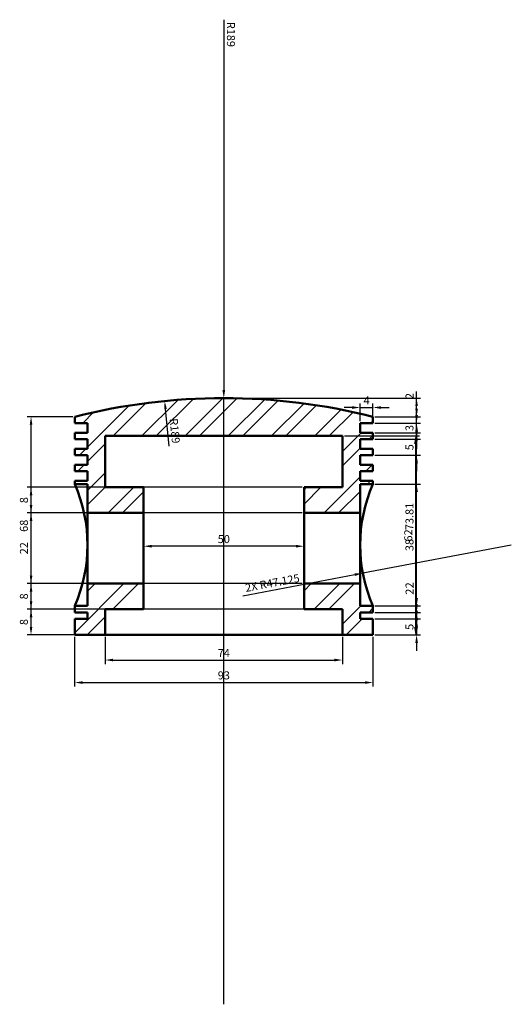
# Model space of a CAD drawing. Units: millimetres. Extents: x 2415 to 2568, y 1198 to 1505.
import ezdxf

# ---------------------------------------------------------------- set-up
doc = ezdxf.new("R2010")
doc.units = ezdxf.units.MM
doc.linetypes.add('CENTER', pattern=[50.8, 31.75, -6.35, 6.35, -6.35])
for name, color, linetype, lineweight in [('M-CNTR', 4, 'CENTER', 18), ('M-DIMS', 2, 'Continuous', 25), ('M-HATC', 8, 'Continuous', 18), ('M-OUTL', 7, 'Continuous', 50)]:
    doc.layers.add(name, color=color, linetype=linetype, lineweight=lineweight)
doc.styles.get("Standard").update_dxf_attribs({"font": 'arial.ttf'})
doc.dimstyles.new('ISO-25', dxfattribs={"dimtxt": 2.5, "dimasz": 2.5, "dimexe": 1.25, "dimexo": 0.625, "dimtad": 1, "dimtxsty": 'Standard', "dimcen": 2.5, "dimadec": 0, "dimazin": 0, "dimtfac": 1, "dimtmove": 0, "dimatfit": 3, "dimfxl": 1, "dimarcsym": 0})

# ---------------------------------------------------------------- blocks, each defined once
blk = doc.blocks.new('*D1')
at = {"layer": 'Defpoints', "color": 0, "transparency": 16777216}
for p in [(2431.97, 1313.29), (2524.97, 1313.29), (2524.97, 1298.42)]:
    blk.add_point(p, dxfattribs=at)
at = {"layer": 'M-DIMS', "color": 0, "lineweight": -2, "transparency": 16777216}
for p, q in [((2431.97, 1312.67), (2431.97, 1297.17)), ((2524.97, 1312.67), (2524.97, 1297.17)), ((2434.47, 1298.42), (2522.47, 1298.42))]:
    blk.add_line(p, q, dxfattribs=at)
at = {"layer": 'M-DIMS', "color": 0, "transparency": 16777216}
for points in [[(2434.47, 1298.84), (2434.47, 1298.01), (2431.97, 1298.42)], [(2522.47, 1298.84), (2522.47, 1298.01), (2524.97, 1298.42)]]:
    blk.add_solid(points, dxfattribs=at)
at = {"layer": 'M-DIMS', "color": 0, "transparency": 16777216, "insert": (2478.47, 1300.33), "char_height": 2.5, "attachment_point": 5}
blk.add_mtext('93', dxfattribs=at)
blk = doc.blocks.new('*D2')
at = {"layer": 'Defpoints', "color": 0, "transparency": 16777216}
for p in [(2441.47, 1313.29), (2515.47, 1313.29), (2515.47, 1305.44)]:
    blk.add_point(p, dxfattribs=at)
at = {"layer": 'M-DIMS', "color": 0, "lineweight": -2, "transparency": 16777216}
for p, q in [((2441.47, 1312.67), (2441.47, 1304.19)), ((2515.47, 1312.67), (2515.47, 1304.19)), ((2443.97, 1305.44), (2512.97, 1305.44))]:
    blk.add_line(p, q, dxfattribs=at)
at = {"layer": 'M-DIMS', "color": 0, "transparency": 16777216}
for points in [[(2443.97, 1305.86), (2443.97, 1305.02), (2441.47, 1305.44)], [(2512.97, 1305.86), (2512.97, 1305.02), (2515.47, 1305.44)]]:
    blk.add_solid(points, dxfattribs=at)
at = {"layer": 'M-DIMS', "color": 0, "transparency": 16777216, "insert": (2478.47, 1307.31), "char_height": 2.5, "attachment_point": 5}
blk.add_mtext('74', dxfattribs=at)
blk = doc.blocks.new('*D3')
at = {"layer": 'Defpoints', "color": 0, "transparency": 16777216}
for p in [(2453.47, 1359.29), (2503.47, 1359.29), (2453.47, 1340.92)]:
    blk.add_point(p, dxfattribs=at)
at = {"layer": 'M-DIMS', "color": 0, "lineweight": -2, "transparency": 16777216}
for p, q in [((2453.47, 1358.67), (2453.47, 1339.67)), ((2503.47, 1358.67), (2503.47, 1339.67)), ((2500.97, 1340.92), (2455.97, 1340.92))]:
    blk.add_line(p, q, dxfattribs=at)
at = {"layer": 'M-DIMS', "color": 0, "transparency": 16777216}
for points in [[(2455.97, 1341.34), (2455.97, 1340.5), (2453.47, 1340.92)], [(2500.97, 1341.34), (2500.97, 1340.5), (2503.47, 1340.92)]]:
    blk.add_solid(points, dxfattribs=at)
at = {"layer": 'M-DIMS', "color": 0, "transparency": 16777216, "insert": (2478.47, 1342.82), "char_height": 2.5, "attachment_point": 5}
blk.add_mtext('50', dxfattribs=at)
blk = doc.blocks.new('*D4')
at = {"layer": 'Defpoints', "color": 0, "transparency": 16777216}
for p in [(2515.47, 1375.29), (2524.97, 1313.29), (2538.21, 1313.29)]:
    blk.add_point(p, dxfattribs=at)
at = {"layer": 'M-DIMS', "color": 0, "lineweight": -2, "transparency": 16777216}
for p, q in [((2516.1, 1375.29), (2539.46, 1375.29)), ((2538.21, 1372.79), (2538.21, 1315.79)), ((2525.6, 1313.29), (2539.46, 1313.29))]:
    blk.add_line(p, q, dxfattribs=at)
at = {"layer": 'M-DIMS', "color": 0, "transparency": 16777216}
for points in [[(2537.79, 1372.79), (2538.62, 1372.79), (2538.21, 1375.29)], [(2537.79, 1315.79), (2538.62, 1315.79), (2538.21, 1313.29)]]:
    blk.add_solid(points, dxfattribs=at)
at = {"layer": 'M-DIMS', "color": 0, "transparency": 16777216, "insert": (2536.3, 1344.29), "char_height": 2.5, "attachment_point": 5, "rotation": 90}
blk.add_mtext('62', dxfattribs=at)
blk = doc.blocks.new('*D5')
at = {"layer": 'Defpoints', "color": 0, "transparency": 16777216}
for p in [(2524.97, 1384.17), (2520.97, 1379.29), (2524.97, 1379.29)]:
    blk.add_point(p, dxfattribs=at)
at = {"layer": 'M-DIMS', "color": 0, "lineweight": -2, "transparency": 16777216}
for p, q in [((2520.97, 1379.92), (2520.97, 1385.42)), ((2524.97, 1379.92), (2524.97, 1385.42)), ((2518.47, 1384.17), (2515.97, 1384.17)), ((2520.97, 1384.17), (2524.97, 1384.17)), ((2527.47, 1384.17), (2529.97, 1384.17))]:
    blk.add_line(p, q, dxfattribs=at)
at = {"layer": 'M-DIMS', "color": 0, "transparency": 16777216}
for points in [[(2518.47, 1384.58), (2518.47, 1383.75), (2520.97, 1384.17)], [(2527.47, 1384.58), (2527.47, 1383.75), (2524.97, 1384.17)]]:
    blk.add_solid(points, dxfattribs=at)
at = {"layer": 'M-DIMS', "color": 0, "transparency": 16777216, "insert": (2522.97, 1386.04), "char_height": 2.5, "attachment_point": 5}
blk.add_mtext('4', dxfattribs=at)
blk = doc.blocks.new('*D6')
at = {"layer": 'Defpoints', "color": 0, "transparency": 16777216}
for p in [(2460.04, 1386.2), (2478.47, 1198.1)]:
    blk.add_point(p, dxfattribs=at)
at = {"layer": 'M-DIMS', "color": 0, "lineweight": -2, "transparency": 16777216}
blk.add_line((2461.42, 1372.1), (2460.29, 1383.71), dxfattribs=at)
at = {"layer": 'M-DIMS', "color": 0, "transparency": 16777216}
blk.add_solid([(2460.7, 1383.75), (2459.87, 1383.67), (2460.04, 1386.2)], dxfattribs=at)
at = {"layer": 'M-DIMS', "color": 0, "transparency": 16777216, "insert": (2462.87, 1376.85), "char_height": 2.5, "attachment_point": 5, "rotation": 275.5966}
blk.add_mtext('R189', dxfattribs=at)
blk = doc.blocks.new('*D7')
at = {"layer": 'Defpoints', "color": 0, "transparency": 16777216}
for p in [(2478.47, 1387.1), (2538.57, 1387.1), (2524.97, 1313.29)]:
    blk.add_point(p, dxfattribs=at)
at = {"layer": 'M-DIMS', "color": 0, "lineweight": -2, "transparency": 16777216}
for p, q in [((2479.1, 1387.1), (2539.82, 1387.1)), ((2538.57, 1315.79), (2538.57, 1384.6)), ((2525.6, 1313.29), (2539.82, 1313.29))]:
    blk.add_line(p, q, dxfattribs=at)
at = {"layer": 'M-DIMS', "color": 0, "transparency": 16777216}
for points in [[(2538.16, 1384.6), (2538.99, 1384.6), (2538.57, 1387.1)], [(2538.16, 1315.79), (2538.99, 1315.79), (2538.57, 1313.29)]]:
    blk.add_solid(points, dxfattribs=at)
at = {"layer": 'M-DIMS', "color": 0, "transparency": 16777216, "insert": (2536.67, 1350.2), "char_height": 2.5, "attachment_point": 5, "rotation": 90}
blk.add_mtext('73.81', dxfattribs=at)
blk = doc.blocks.new('*D8')
at = {"layer": 'Defpoints', "color": 0, "transparency": 16777216}
for p in [(2418.37, 1381.29), (2431.97, 1381.29), (2431.97, 1313.29)]:
    blk.add_point(p, dxfattribs=at)
at = {"layer": 'M-DIMS', "color": 0, "lineweight": -2, "transparency": 16777216}
for p, q in [((2431.35, 1381.29), (2417.12, 1381.29)), ((2418.37, 1315.79), (2418.37, 1378.79)), ((2431.35, 1313.29), (2417.12, 1313.29))]:
    blk.add_line(p, q, dxfattribs=at)
at = {"layer": 'M-DIMS', "color": 0, "transparency": 16777216}
for points in [[(2417.96, 1378.79), (2418.79, 1378.79), (2418.37, 1381.29)], [(2417.96, 1315.79), (2418.79, 1315.79), (2418.37, 1313.29)]]:
    blk.add_solid(points, dxfattribs=at)
at = {"layer": 'M-DIMS', "color": 0, "transparency": 16777216, "insert": (2416.47, 1347.29), "char_height": 2.5, "attachment_point": 5, "rotation": 90}
blk.add_mtext('68', dxfattribs=at)
blk = doc.blocks.new('*D9')
at = {"layer": 'Defpoints', "color": 0, "transparency": 16777216}
for p in [(2524.97, 1318.29), (2538.57, 1318.29), (2524.97, 1313.29)]:
    blk.add_point(p, dxfattribs=at)
at = {"layer": 'M-DIMS', "color": 0, "lineweight": -2, "transparency": 16777216}
for p, q in [((2538.57, 1320.79), (2538.57, 1323.29)), ((2525.6, 1318.29), (2539.82, 1318.29)), ((2538.57, 1313.29), (2538.57, 1318.29)), ((2525.6, 1313.29), (2539.82, 1313.29)), ((2538.57, 1310.79), (2538.57, 1308.29))]:
    blk.add_line(p, q, dxfattribs=at)
at = {"layer": 'M-DIMS', "color": 0, "transparency": 16777216}
for points in [[(2538.16, 1320.79), (2538.99, 1320.79), (2538.57, 1318.29)], [(2538.16, 1310.79), (2538.99, 1310.79), (2538.57, 1313.29)]]:
    blk.add_solid(points, dxfattribs=at)
at = {"layer": 'M-DIMS', "color": 0, "transparency": 16777216, "insert": (2536.68, 1315.79), "char_height": 2.5, "attachment_point": 5, "rotation": 90}
blk.add_mtext('5', dxfattribs=at)
blk = doc.blocks.new('*D10')
at = {"layer": 'Defpoints', "color": 0, "transparency": 16777216}
for p in [(2524.97, 1320.29), (2538.57, 1320.29), (2524.97, 1318.29)]:
    blk.add_point(p, dxfattribs=at)
at = {"layer": 'M-DIMS', "color": 0, "lineweight": -2, "transparency": 16777216}
for p, q in [((2538.57, 1322.79), (2538.57, 1328.2)), ((2525.6, 1320.29), (2539.82, 1320.29)), ((2538.57, 1318.29), (2538.57, 1320.29)), ((2525.6, 1318.29), (2539.82, 1318.29)), ((2538.57, 1315.79), (2538.57, 1313.29))]:
    blk.add_line(p, q, dxfattribs=at)
at = {"layer": 'M-DIMS', "color": 0, "transparency": 16777216}
for points in [[(2538.16, 1322.79), (2538.99, 1322.79), (2538.57, 1320.29)], [(2538.16, 1315.79), (2538.99, 1315.79), (2538.57, 1318.29)]]:
    blk.add_solid(points, dxfattribs=at)
at = {"layer": 'M-DIMS', "color": 0, "transparency": 16777216, "insert": (2536.69, 1326.74), "char_height": 2.5, "attachment_point": 5, "rotation": 90}
blk.add_mtext('2', dxfattribs=at)
blk = doc.blocks.new('*D11')
at = {"layer": 'Defpoints', "color": 0, "transparency": 16777216}
for p in [(2524.97, 1322.29), (2524.97, 1320.29), (2538.57, 1322.29)]:
    blk.add_point(p, dxfattribs=at)
at = {"layer": 'M-DIMS', "color": 0, "lineweight": -2, "transparency": 16777216}
for p, q in [((2538.57, 1324.79), (2538.57, 1330.2)), ((2525.6, 1322.29), (2539.82, 1322.29)), ((2525.6, 1320.29), (2539.82, 1320.29)), ((2538.57, 1320.29), (2538.57, 1322.29)), ((2538.57, 1317.79), (2538.57, 1315.29))]:
    blk.add_line(p, q, dxfattribs=at)
at = {"layer": 'M-DIMS', "color": 0, "transparency": 16777216}
for points in [[(2538.16, 1324.79), (2538.99, 1324.79), (2538.57, 1322.29)], [(2538.16, 1317.79), (2538.99, 1317.79), (2538.57, 1320.29)]]:
    blk.add_solid(points, dxfattribs=at)
at = {"layer": 'M-DIMS', "color": 0, "transparency": 16777216, "insert": (2536.69, 1328.74), "char_height": 2.5, "attachment_point": 5, "rotation": 90}
blk.add_mtext('2', dxfattribs=at)
blk = doc.blocks.new('*D12')
at = {"layer": 'Defpoints', "color": 0, "transparency": 16777216}
for p in [(2524.97, 1360.29), (2538.57, 1360.29), (2524.97, 1322.29)]:
    blk.add_point(p, dxfattribs=at)
at = {"layer": 'M-DIMS', "color": 0, "lineweight": -2, "transparency": 16777216}
for p, q in [((2525.6, 1360.29), (2539.82, 1360.29)), ((2538.57, 1324.79), (2538.57, 1357.79)), ((2525.6, 1322.29), (2539.82, 1322.29))]:
    blk.add_line(p, q, dxfattribs=at)
at = {"layer": 'M-DIMS', "color": 0, "transparency": 16777216}
for points in [[(2538.16, 1357.79), (2538.99, 1357.79), (2538.57, 1360.29)], [(2538.16, 1324.79), (2538.99, 1324.79), (2538.57, 1322.29)]]:
    blk.add_solid(points, dxfattribs=at)
at = {"layer": 'M-DIMS', "color": 0, "transparency": 16777216, "insert": (2536.67, 1341.29), "char_height": 2.5, "attachment_point": 5, "rotation": 90}
blk.add_mtext('38', dxfattribs=at)
blk = doc.blocks.new('*D13')
at = {"layer": 'Defpoints', "color": 0, "transparency": 16777216}
for p in [(2524.97, 1374.29), (2538.57, 1374.29), (2524.97, 1369.29)]:
    blk.add_point(p, dxfattribs=at)
at = {"layer": 'M-DIMS', "color": 0, "lineweight": -2, "transparency": 16777216}
for p, q in [((2538.57, 1376.79), (2538.57, 1379.29)), ((2525.6, 1374.29), (2539.82, 1374.29)), ((2538.57, 1369.29), (2538.57, 1374.29)), ((2525.6, 1369.29), (2539.82, 1369.29)), ((2538.57, 1366.79), (2538.57, 1364.29))]:
    blk.add_line(p, q, dxfattribs=at)
at = {"layer": 'M-DIMS', "color": 0, "transparency": 16777216}
for points in [[(2538.16, 1376.79), (2538.99, 1376.79), (2538.57, 1374.29)], [(2538.16, 1366.79), (2538.99, 1366.79), (2538.57, 1369.29)]]:
    blk.add_solid(points, dxfattribs=at)
at = {"layer": 'M-DIMS', "color": 0, "transparency": 16777216, "insert": (2536.68, 1371.79), "char_height": 2.5, "attachment_point": 5, "rotation": 90}
blk.add_mtext('5', dxfattribs=at)
blk = doc.blocks.new('*D14')
at = {"layer": 'Defpoints', "color": 0, "transparency": 16777216}
for p in [(2524.97, 1379.29), (2538.57, 1379.29), (2524.97, 1376.29)]:
    blk.add_point(p, dxfattribs=at)
at = {"layer": 'M-DIMS', "color": 0, "lineweight": -2, "transparency": 16777216}
for p, q in [((2538.57, 1381.79), (2538.57, 1384.29)), ((2525.6, 1379.29), (2539.82, 1379.29)), ((2538.57, 1376.29), (2538.57, 1379.29)), ((2525.6, 1376.29), (2539.82, 1376.29)), ((2538.57, 1373.79), (2538.57, 1371.29))]:
    blk.add_line(p, q, dxfattribs=at)
at = {"layer": 'M-DIMS', "color": 0, "transparency": 16777216}
for points in [[(2538.16, 1381.79), (2538.99, 1381.79), (2538.57, 1379.29)], [(2538.16, 1373.79), (2538.99, 1373.79), (2538.57, 1376.29)]]:
    blk.add_solid(points, dxfattribs=at)
at = {"layer": 'M-DIMS', "color": 0, "transparency": 16777216, "insert": (2536.67, 1377.79), "char_height": 2.5, "attachment_point": 5, "rotation": 90}
blk.add_mtext('3', dxfattribs=at)
blk = doc.blocks.new('*D15')
at = {"layer": 'Defpoints', "color": 0, "transparency": 16777216}
for p in [(2524.97, 1381.29), (2524.97, 1379.29), (2538.57, 1381.29)]:
    blk.add_point(p, dxfattribs=at)
at = {"layer": 'M-DIMS', "color": 0, "lineweight": -2, "transparency": 16777216}
for p, q in [((2538.57, 1383.79), (2538.57, 1389.2)), ((2525.6, 1381.29), (2539.82, 1381.29)), ((2525.6, 1379.29), (2539.82, 1379.29)), ((2538.57, 1379.29), (2538.57, 1381.29)), ((2538.57, 1376.79), (2538.57, 1374.29))]:
    blk.add_line(p, q, dxfattribs=at)
at = {"layer": 'M-DIMS', "color": 0, "transparency": 16777216}
for points in [[(2538.16, 1383.79), (2538.99, 1383.79), (2538.57, 1381.29)], [(2538.16, 1376.79), (2538.99, 1376.79), (2538.57, 1379.29)]]:
    blk.add_solid(points, dxfattribs=at)
at = {"layer": 'M-DIMS', "color": 0, "transparency": 16777216, "insert": (2536.69, 1387.74), "char_height": 2.5, "attachment_point": 5, "rotation": 90}
blk.add_mtext('2', dxfattribs=at)
blk = doc.blocks.new('*D16')
at = {"layer": 'Defpoints', "color": 0, "transparency": 16777216}
for p in [(2418.37, 1321.29), (2515.47, 1321.29), (2515.47, 1313.29)]:
    blk.add_point(p, dxfattribs=at)
at = {"layer": 'M-DIMS', "color": 0, "lineweight": -2, "transparency": 16777216}
for p, q in [((2514.85, 1321.29), (2417.12, 1321.29)), ((2418.37, 1315.79), (2418.37, 1318.79)), ((2514.85, 1313.29), (2417.12, 1313.29))]:
    blk.add_line(p, q, dxfattribs=at)
at = {"layer": 'M-DIMS', "color": 0, "transparency": 16777216}
for points in [[(2417.96, 1318.79), (2418.79, 1318.79), (2418.37, 1321.29)], [(2417.96, 1315.79), (2418.79, 1315.79), (2418.37, 1313.29)]]:
    blk.add_solid(points, dxfattribs=at)
at = {"layer": 'M-DIMS', "color": 0, "transparency": 16777216, "insert": (2416.47, 1317.29), "char_height": 2.5, "attachment_point": 5, "rotation": 90}
blk.add_mtext('8', dxfattribs=at)
blk = doc.blocks.new('*D17')
at = {"layer": 'Defpoints', "color": 0, "transparency": 16777216}
for p in [(2418.37, 1329.29), (2503.47, 1329.29), (2503.47, 1321.29)]:
    blk.add_point(p, dxfattribs=at)
at = {"layer": 'M-DIMS', "color": 0, "lineweight": -2, "transparency": 16777216}
for p, q in [((2502.85, 1329.29), (2417.12, 1329.29)), ((2418.37, 1323.79), (2418.37, 1326.79)), ((2502.85, 1321.29), (2417.12, 1321.29))]:
    blk.add_line(p, q, dxfattribs=at)
at = {"layer": 'M-DIMS', "color": 0, "transparency": 16777216}
for points in [[(2417.96, 1326.79), (2418.79, 1326.79), (2418.37, 1329.29)], [(2417.96, 1323.79), (2418.79, 1323.79), (2418.37, 1321.29)]]:
    blk.add_solid(points, dxfattribs=at)
at = {"layer": 'M-DIMS', "color": 0, "transparency": 16777216, "insert": (2416.47, 1325.29), "char_height": 2.5, "attachment_point": 5, "rotation": 90}
blk.add_mtext('8', dxfattribs=at)
blk = doc.blocks.new('*D18')
at = {"layer": 'Defpoints', "color": 0, "transparency": 16777216}
for p in [(2418.37, 1351.29), (2503.47, 1351.29), (2503.47, 1329.29)]:
    blk.add_point(p, dxfattribs=at)
at = {"layer": 'M-DIMS', "color": 0, "lineweight": -2, "transparency": 16777216}
for p, q in [((2502.85, 1351.29), (2417.12, 1351.29)), ((2418.37, 1331.79), (2418.37, 1348.79)), ((2502.85, 1329.29), (2417.12, 1329.29))]:
    blk.add_line(p, q, dxfattribs=at)
at = {"layer": 'M-DIMS', "color": 0, "transparency": 16777216}
for points in [[(2417.96, 1348.79), (2418.79, 1348.79), (2418.37, 1351.29)], [(2417.96, 1331.79), (2418.79, 1331.79), (2418.37, 1329.29)]]:
    blk.add_solid(points, dxfattribs=at)
at = {"layer": 'M-DIMS', "color": 0, "transparency": 16777216, "insert": (2416.49, 1340.29), "char_height": 2.5, "attachment_point": 5, "rotation": 90}
blk.add_mtext('22', dxfattribs=at)
blk = doc.blocks.new('*D19')
at = {"layer": 'Defpoints', "color": 0, "transparency": 16777216}
for p in [(2418.37, 1359.29), (2503.47, 1359.29), (2503.47, 1351.29)]:
    blk.add_point(p, dxfattribs=at)
at = {"layer": 'M-DIMS', "color": 0, "lineweight": -2, "transparency": 16777216}
for p, q in [((2502.85, 1359.29), (2417.12, 1359.29)), ((2418.37, 1353.79), (2418.37, 1356.79)), ((2502.85, 1351.29), (2417.12, 1351.29))]:
    blk.add_line(p, q, dxfattribs=at)
at = {"layer": 'M-DIMS', "color": 0, "transparency": 16777216}
for points in [[(2417.96, 1356.79), (2418.79, 1356.79), (2418.37, 1359.29)], [(2417.96, 1353.79), (2418.79, 1353.79), (2418.37, 1351.29)]]:
    blk.add_solid(points, dxfattribs=at)
at = {"layer": 'M-DIMS', "color": 0, "transparency": 16777216, "insert": (2416.47, 1355.29), "char_height": 2.5, "attachment_point": 5, "rotation": 90}
blk.add_mtext('8', dxfattribs=at)
blk = doc.blocks.new('*D20')
at = {"layer": 'Defpoints', "color": 0, "transparency": 16777216}
for p in [(2478.47, 1387.1), (2478.47, 1198.1)]:
    blk.add_point(p, dxfattribs=at)
at = {"layer": 'M-DIMS', "color": 0, "lineweight": -2, "transparency": 16777216}
for p, q in [((2478.47, 1505.09), (2478.47, 1389.6)), ((2478.47, 1198.1), (2478.47, 1387.1))]:
    blk.add_line(p, q, dxfattribs=at)
at = {"layer": 'M-DIMS', "color": 0, "transparency": 16777216}
blk.add_solid([(2478.89, 1389.6), (2478.05, 1389.6), (2478.47, 1387.1)], dxfattribs=at)
at = {"layer": 'M-DIMS', "color": 0, "transparency": 16777216, "insert": (2480.37, 1500.5), "char_height": 2.5, "attachment_point": 5, "rotation": 270.0011}
blk.add_mtext('R189', dxfattribs=at)
blk = doc.blocks.new('*D21')
at = {"layer": 'Defpoints', "color": 0, "transparency": 16777216}
for p in [(2568.1, 1341.29), (2521.79, 1332.54)]:
    blk.add_point(p, dxfattribs=at)
at = {"layer": 'M-DIMS', "color": 0, "lineweight": -2, "transparency": 16777216}
for p, q in [((2568.1, 1341.29), (2521.79, 1332.54)), ((2484.45, 1325.48), (2519.34, 1332.07))]:
    blk.add_line(p, q, dxfattribs=at)
at = {"layer": 'M-DIMS', "color": 0, "transparency": 16777216}
blk.add_solid([(2519.26, 1332.48), (2519.41, 1331.66), (2521.79, 1332.54)], dxfattribs=at)
at = {"layer": 'M-DIMS', "color": 0, "transparency": 16777216, "insert": (2493.66, 1329.15), "char_height": 2.5, "attachment_point": 5, "rotation": 10.7069}
blk.add_mtext('2X R47.125', dxfattribs=at)

msp = doc.modelspace()

# ---------------------------------------------------------------- hatches: boundary and pattern name
at = {"layer": 'M-HATC'}
h = msp.add_hatch(dxfattribs=at)
h.set_pattern_fill('ANSI32', color=256)
h.paths.add_polyline_path([(2520.9736, 1329.2918), (2503.4736, 1329.2918), (2503.4736, 1321.2918), (2515.4736, 1321.2918), (2515.4736, 1313.2918), (2524.9736, 1313.2918), (2524.9736, 1318.2918), (2520.9736, 1318.2918), (2520.9736, 1320.2918), (2524.9736, 1320.2918), (2524.9736, 1322.2918), (2520.9736, 1322.2918)])
h.paths.add_polyline_path([(2520.9736, 1360.2918), (2524.9736, 1360.2918), (2524.9736, 1361.2918), (2520.9736, 1361.2918), (2520.9736, 1364.2918), (2524.9736, 1364.2918), (2524.9736, 1366.2918), (2520.9736, 1366.2918), (2520.9736, 1369.2918), (2524.9736, 1369.2918), (2524.9736, 1371.2918), (2520.9736, 1371.2918), (2520.9736, 1374.2918), (2524.9736, 1374.2918), (2524.9736, 1376.2918), (2520.9736, 1376.2918), (2520.9736, 1379.2918), (2524.9736, 1379.2918), (2524.9736, 1381.2918, 0.12493603), (2431.9736, 1381.2918), (2431.9736, 1379.2918), (2435.9736, 1379.2918), (2435.9736, 1376.2918), (2431.9736, 1376.2918), (2431.9736, 1374.2918), (2435.9736, 1374.2918), (2435.9736, 1371.2918), (2431.9736, 1371.2918), (2431.9736, 1369.2918), (2435.9736, 1369.2918), (2435.9736, 1366.2918), (2431.9736, 1366.2918), (2431.9736, 1364.2918), (2435.9736, 1364.2918), (2435.9736, 1361.2918), (2431.9736, 1361.2918), (2431.9736, 1360.2918), (2435.9736, 1360.2918), (2435.9736, 1351.2918), (2453.4736, 1351.2918), (2453.4736, 1359.2918), (2441.4736, 1359.2918), (2441.4736, 1375.2918), (2478.4736, 1375.2918), (2515.4736, 1375.2918), (2515.4736, 1359.2918), (2503.4736, 1359.2918), (2503.4736, 1351.2918), (2520.9736, 1351.2918)])
h.paths.add_polyline_path([(2453.4736, 1329.2918), (2435.9736, 1329.2918), (2435.9736, 1322.2918), (2431.9736, 1322.2918), (2431.9736, 1320.2918), (2435.9736, 1320.2918), (2435.9736, 1318.2918), (2431.9736, 1318.2918), (2431.9736, 1313.2918), (2441.4736, 1313.2918), (2441.4736, 1321.2918), (2453.4736, 1321.2918)])

# ---------------------------------------------------------------- linework, layer by layer
at = {"layer": 'M-CNTR'}
msp.add_line((2478.4736, 1313.2918), (2478.4736, 1375.2918), dxfattribs=at)
at = {"layer": 'M-OUTL'}
for p, q in [((2431.9736, 1379.2918), (2431.9736, 1381.2918)), ((2435.9736, 1379.2918), (2431.9736, 1379.2918)), ((2435.9736, 1376.2918), (2435.9736, 1379.2918)), ((2520.9736, 1376.2918), (2520.9736, 1379.2918)), ((2520.9736, 1379.2918), (2524.9736, 1379.2918)), ((2524.9736, 1379.2918), (2524.9736, 1381.2918)), ((2431.9736, 1374.2918), (2431.9736, 1376.2918)), ((2431.9736, 1376.2918), (2435.9736, 1376.2918)), ((2524.9736, 1376.2918), (2520.9736, 1376.2918)), ((2524.9736, 1374.2918), (2524.9736, 1376.2918)), ((2435.9736, 1374.2918), (2431.9736, 1374.2918)), ((2435.9736, 1371.2918), (2435.9736, 1374.2918)), ((2441.4736, 1359.2918), (2441.4736, 1375.2918)), ((2441.4736, 1375.2918), (2478.4736, 1375.2918)), ((2515.4736, 1375.2918), (2478.4736, 1375.2918)), ((2515.4736, 1359.2918), (2515.4736, 1375.2918)), ((2520.9736, 1371.2918), (2520.9736, 1374.2918)), ((2520.9736, 1374.2918), (2524.9736, 1374.2918)), ((2431.9736, 1369.2918), (2431.9736, 1371.2918)), ((2431.9736, 1371.2918), (2435.9736, 1371.2918)), ((2435.9736, 1369.2918), (2431.9736, 1369.2918)), ((2435.9736, 1366.2918), (2435.9736, 1369.2918)), ((2524.9736, 1371.2918), (2520.9736, 1371.2918)), ((2520.9736, 1366.2918), (2520.9736, 1369.2918)), ((2520.9736, 1369.2918), (2524.9736, 1369.2918)), ((2524.9736, 1369.2918), (2524.9736, 1371.2918)), ((2431.9736, 1364.2918), (2431.9736, 1366.2918)), ((2431.9736, 1366.2918), (2435.9736, 1366.2918)), ((2524.9736, 1366.2918), (2520.9736, 1366.2918)), ((2524.9736, 1364.2918), (2524.9736, 1366.2918)), ((2435.9736, 1364.2918), (2431.9736, 1364.2918)), ((2435.9736, 1361.2918), (2435.9736, 1364.2918)), ((2520.9736, 1361.2918), (2520.9736, 1364.2918)), ((2520.9736, 1364.2918), (2524.9736, 1364.2918)), ((2431.9736, 1361.2918), (2435.9736, 1361.2918)), ((2431.9736, 1360.2918), (2431.9736, 1361.2918)), ((2435.9736, 1360.2918), (2431.9736, 1360.2918)), ((2435.9736, 1322.2918), (2435.9736, 1360.2918)), ((2524.9736, 1361.2918), (2520.9736, 1361.2918)), ((2520.9736, 1360.2918), (2524.9736, 1360.2918)), ((2520.9736, 1322.2918), (2520.9736, 1360.2918)), ((2524.9736, 1360.2918), (2524.9736, 1361.2918)), ((2453.4736, 1359.2918), (2441.4736, 1359.2918)), ((2453.4736, 1321.2918), (2453.4736, 1359.2918)), ((2503.4736, 1321.2918), (2503.4736, 1359.2918)), ((2503.4736, 1359.2918), (2515.4736, 1359.2918)), ((2453.4736, 1351.2918), (2435.9736, 1351.2918)), ((2503.4736, 1351.2918), (2520.9736, 1351.2918)), ((2435.9736, 1329.2918), (2453.4736, 1329.2918)), ((2520.9736, 1329.2918), (2503.4736, 1329.2918)), ((2431.9736, 1320.2918), (2431.9736, 1322.2918)), ((2431.9736, 1322.2918), (2435.9736, 1322.2918)), ((2435.9736, 1320.2918), (2431.9736, 1320.2918)), ((2435.9736, 1318.2918), (2435.9736, 1320.2918)), ((2441.4736, 1313.2918), (2441.4736, 1321.2918)), ((2441.4736, 1321.2918), (2453.4736, 1321.2918)), ((2515.4736, 1321.2918), (2503.4736, 1321.2918)), ((2515.4736, 1313.2918), (2515.4736, 1321.2918)), ((2524.9736, 1322.2918), (2520.9736, 1322.2918)), ((2520.9736, 1318.2918), (2520.9736, 1320.2918)), ((2520.9736, 1320.2918), (2524.9736, 1320.2918)), ((2524.9736, 1320.2918), (2524.9736, 1322.2918)), ((2431.9736, 1313.2918), (2431.9736, 1318.2918)), ((2431.9736, 1318.2918), (2435.9736, 1318.2918)), ((2524.9736, 1318.2918), (2520.9736, 1318.2918)), ((2524.9736, 1313.2918), (2524.9736, 1318.2918)), ((2441.4736, 1313.2918), (2431.9736, 1313.2918)), ((2441.4736, 1313.2918), (2515.4736, 1313.2918)), ((2515.4736, 1313.2918), (2524.9736, 1313.2918))]:
    msp.add_line(p, q, dxfattribs=at)
for centre, radius, start, end in [((2478.4736, 1198.1013), 189, 75.757185, 104.242815), ((2388.8486, 1341.2918), 47.125, 336.222684, 23.777316), ((2568.0986, 1341.2918), 47.125, 156.222684, 203.777316)]:
    msp.add_arc(centre, radius, start, end, dxfattribs=at)

# ---------------------------------------------------------------- dimensions: what is measured, and where the dimension line sits
at = {"layer": 'M-DIMS'}
for mpoint, override, picture, middle in [((2478.47, 1387.1013), {"dimdec": 0, "dimlfac": 1, "dimrnd": 0, "dimzin": 0, "dimdsep": 46, "dimlunit": 2}, '*D20', (2478.4678, 1500.5013)), ((2460.0416, 1386.2004), {"dimclrd": 0, "dimclre": 0, "dimclrt": 0}, '*D6', (2460.9765, 1376.6605))]:
    dim = msp.add_radius_dim(center=(2478.4736, 1198.1013), mpoint=mpoint, dimstyle='ISO-25', override=override, dxfattribs=at)
    dim.commit()
    dim.dimension.update_dxf_attribs({"geometry": picture, "text_midpoint": middle, "dimtype": 164})
for base, p1, p2, picture, middle in [((2524.9736, 1384.1667), (2520.9736, 1379.2918), (2524.9736, 1379.2918), '*D5', (2522.9736, 1386.0417)), ((2453.4736, 1340.9215), (2503.4736, 1359.2918), (2453.4736, 1359.2918), '*D3', (2478.4736, 1342.823)), ((2524.9736, 1298.4238), (2431.9736, 1313.2918), (2524.9736, 1313.2918), '*D1', (2478.4736, 1300.3261)), ((2515.4736, 1305.44), (2441.4736, 1313.2918), (2515.4736, 1313.2918), '*D2', (2478.4736, 1307.315))]:
    dim = msp.add_linear_dim(base=base, p1=p1, p2=p2, dimstyle='ISO-25', override={"dimclrd": 0, "dimclre": 0, "dimclrt": 0}, dxfattribs=at)
    dim.commit()
    dim.dimension.update_dxf_attribs({"geometry": picture, "text_midpoint": middle})
for base, p1, p2, override, picture, middle in [((2538.5736, 1381.2918), (2524.9736, 1379.2918), (2524.9736, 1381.2918), {"dimdec": 0, "dimlfac": 1, "dimrnd": 0, "dimzin": 0, "dimdsep": 46, "dimlunit": 2}, '*D15', (2536.6935, 1387.7447)), ((2538.5736, 1387.1013), (2524.9736, 1313.2918), (2478.4736, 1387.1013), {"dimdec": 2, "dimlfac": 1, "dimrnd": 0, "dimzin": 0, "dimdsep": 46, "dimlunit": 2}, '*D7', (2536.6714, 1350.1966)), ((2538.5736, 1379.2918), (2524.9736, 1376.2918), (2524.9736, 1379.2918), {"dimdec": 0, "dimlfac": 1, "dimrnd": 0, "dimzin": 0, "dimdsep": 46, "dimlunit": 2}, '*D14', (2536.6714, 1377.7918)), ((2418.3736, 1381.2918), (2431.9736, 1313.2918), (2431.9736, 1381.2918), {"dimdec": 0, "dimlfac": 1, "dimrnd": 0, "dimzin": 0, "dimdsep": 46, "dimlunit": 2}, '*D8', (2416.4722, 1347.2918)), ((2538.5736, 1374.2918), (2524.9736, 1369.2918), (2524.9736, 1374.2918), {"dimdec": 0, "dimlfac": 1, "dimrnd": 0, "dimzin": 0, "dimdsep": 46, "dimlunit": 2}, '*D13', (2536.6773, 1371.7918)), ((2538.2053, 1313.2918), (2515.4736, 1375.2918), (2524.9736, 1313.2918), {"dimclrd": 0, "dimclre": 0, "dimclrt": 0}, '*D4', (2536.3038, 1344.2918)), ((2538.5736, 1360.2918), (2524.9736, 1322.2918), (2524.9736, 1360.2918), {"dimdec": 0, "dimlfac": 1, "dimrnd": 0, "dimzin": 0, "dimdsep": 46, "dimlunit": 2}, '*D12', (2536.6714, 1341.2918)), ((2418.3736, 1359.2918), (2503.4736, 1351.2918), (2503.4736, 1359.2918), {"dimdec": 0, "dimlfac": 1, "dimrnd": 0, "dimzin": 0, "dimdsep": 46, "dimlunit": 2}, '*D19', (2416.4722, 1355.2918)), ((2418.3736, 1351.2918), (2503.4736, 1329.2918), (2503.4736, 1351.2918), {"dimdec": 0, "dimlfac": 1, "dimrnd": 0, "dimzin": 0, "dimdsep": 46, "dimlunit": 2}, '*D18', (2416.4935, 1340.2918)), ((2418.3736, 1329.2918), (2503.4736, 1321.2918), (2503.4736, 1329.2918), {"dimdec": 0, "dimlfac": 1, "dimrnd": 0, "dimzin": 0, "dimdsep": 46, "dimlunit": 2}, '*D17', (2416.4722, 1325.2918)), ((2538.5736, 1322.2918), (2524.9736, 1320.2918), (2524.9736, 1322.2918), {"dimdec": 0, "dimlfac": 1, "dimrnd": 0, "dimzin": 0, "dimdsep": 46, "dimlunit": 2}, '*D11', (2536.6935, 1328.7447)), ((2538.5736, 1320.2918), (2524.9736, 1318.2918), (2524.9736, 1320.2918), {"dimdec": 0, "dimlfac": 1, "dimrnd": 0, "dimzin": 0, "dimdsep": 46, "dimlunit": 2}, '*D10', (2536.6935, 1326.7447)), ((2538.5736, 1318.2918), (2524.9736, 1313.2918), (2524.9736, 1318.2918), {"dimdec": 0, "dimlfac": 1, "dimrnd": 0, "dimzin": 0, "dimdsep": 46, "dimlunit": 2}, '*D9', (2536.6773, 1315.7918)), ((2418.3736, 1321.2918), (2515.4736, 1313.2918), (2515.4736, 1321.2918), {"dimdec": 0, "dimlfac": 1, "dimrnd": 0, "dimzin": 0, "dimdsep": 46, "dimlunit": 2}, '*D16', (2416.4722, 1317.2918))]:
    dim = msp.add_linear_dim(base=base, p1=p1, p2=p2, angle=90, dimstyle='ISO-25', override=override, dxfattribs=at)
    dim.commit()
    dim.dimension.update_dxf_attribs({"geometry": picture, "text_midpoint": middle})
dim = msp.add_radius_dim(center=(2568.0986, 1341.2918), mpoint=(2521.7941, 1332.5367), text='2X <>', dimstyle='ISO-25', override={"dimdec": 3, "dimlfac": 1, "dimrnd": 0, "dimzin": 0, "dimdsep": 46, "dimlunit": 2}, dxfattribs=at)
dim.commit()
dim.dimension.update_dxf_attribs({"geometry": '*D21', "text_midpoint": (2494.0113, 1327.2836), "dimtype": 164})

doc.saveas('drawing.dxf')
